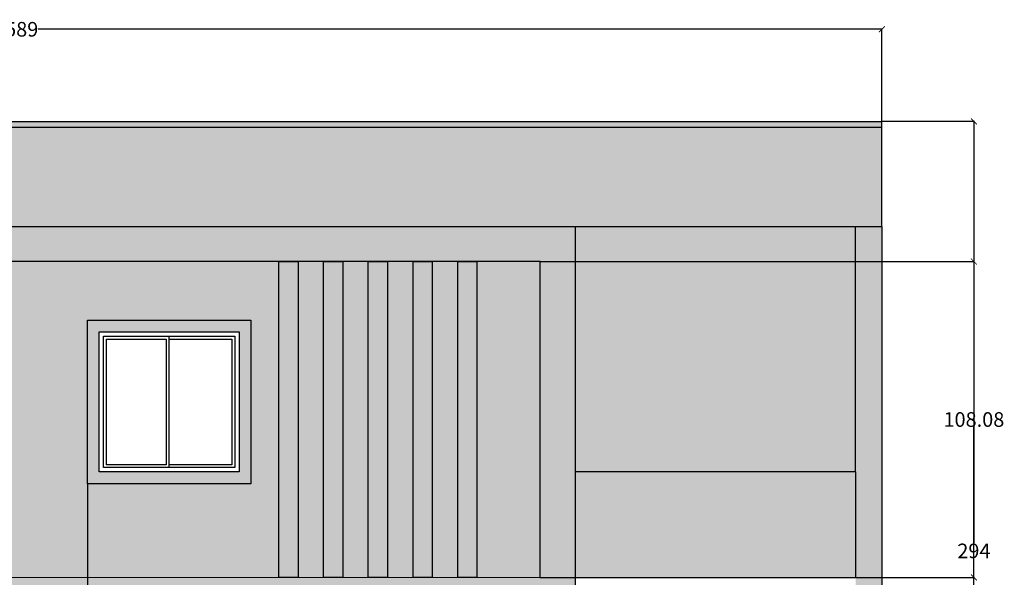
# Model space of a CAD drawing. Units: inches. Extents: x 1455 to 5994, y -182 to 2370.
# Tile 7 of 8: x 4579 to 4916, y 49 to 240. Entities that reach past the tile are written whole.
import ezdxf

# ---------------------------------------------------------------- set-up
doc = ezdxf.new("R2010")
doc.units = ezdxf.units.IN
doc.header["$MEASUREMENT"] = 0
for name, color, linetype, lineweight in [('A-ANNO-DIMS', 2, 'Continuous', 18), ('A-ELEV', 7, 'Continuous', 25), ('A-ELEV-PATT', 8, 'Continuous', 13)]:
    doc.layers.add(name, color=color, linetype=linetype, lineweight=lineweight)
doc.styles.get("Standard").update_dxf_attribs({"font": 'arial.ttf'})
doc.dimstyles.get("Standard").update_dxf_attribs({"dimtxt": 5, "dimasz": 2, "dimexe": 0.18, "dimexo": 0.0625, "dimgap": 0.09, "dimtad": 0, "dimtih": 1, "dimtoh": 1, "dimdec": 1, "dimzin": 0, "dimdsep": 46, "dimlunit": 3, "dimtxsty": 'Standard', "dimblk": 'ARCHTICK', "dimcen": 0.09, "dimadec": 0, "dimazin": 0, "dimtfac": 1, "dimtdec": 1, "dimtofl": 0, "dimtmove": 0, "dimatfit": 3, "dimfxl": 1, "dimtolj": 1, "dimtzin": 0, "dimarcsym": 0})

# ---------------------------------------------------------------- blocks, each defined once
blk = doc.blocks.new('*U8')
for p, q in [((1.5, 1.5), (1.5, 46.5)), ((1.5, 46.5), (24, 46.5)), ((24, 1.5), (24, 46.5)), ((24, 46.5), (46.5, 46.5)), ((46.5, 46.5), (46.5, 1.5)), ((24, 1.5), (1.5, 1.5)), ((46.5, 1.5), (24, 1.5))]:
    blk.add_line(p, q)
blk.add_lwpolyline([(0, 0), (0, 48), (48, 48), (48, 0)], close=True)
for points in [[(23, 45.5), (23, 2.5), (2.5, 2.5), (2.5, 45.5), (23, 45.5)], [(24, 45.5), (45.5, 45.5), (45.5, 2.5), (24, 2.5)]]:
    blk.add_lwpolyline(points)
blk = doc.blocks.new('_ArchTick')
at = {"color": 0, "linetype": 'ByBlock', "const_width": 0.15}
blk.add_lwpolyline([(-0.5, -0.5), (0.5, 0.5)], dxfattribs=at)
blk = doc.blocks.new('*D84')
at = {"layer": 'A-ANNO-DIMS', "color": 0, "lineweight": -2, "transparency": 16777216}
for p, q in [((4873.75, 205.1), (4905.37, 205.1)), ((4905.19, 205.1), (4905.19, 60.74)), ((4905.19, -88.9), (4905.19, 55.45)), ((4873.75, -88.9), (4905.37, -88.9))]:
    blk.add_line(p, q, dxfattribs=at)
at = {"layer": 'Defpoints', "color": 0, "lineweight": 25, "transparency": 16777216}
for p in [(4873.69, 205.1), (4905.19, 205.1), (4873.69, -88.9)]:
    blk.add_point(p, dxfattribs=at)
at = {"layer": 'A-ANNO-DIMS', "color": 0, "lineweight": -2, "transparency": 16777216, "xscale": 2, "yscale": 2, "zscale": 2}
for p, rotation in [((4905.19, 205.1), 90), ((4905.19, -88.9), 270)]:
    blk.add_blockref('_ArchTick', p, dxfattribs=dict(at, rotation=rotation))
at = {"layer": 'A-ANNO-DIMS', "color": 0, "transparency": 16777216, "insert": (4905.19, 58.1), "char_height": 5, "attachment_point": 5}
blk.add_mtext('\\A1;294', dxfattribs=at)
blk = doc.blocks.new('*D86')
at = {"layer": 'A-ANNO-DIMS', "color": 0, "lineweight": -2, "transparency": 16777216}
for p, q in [((4284.69, 205.16), (4284.69, 236.78)), ((4284.69, 236.6), (4573.57, 236.6)), ((4873.69, 236.6), (4584.81, 236.6)), ((4873.69, 205.16), (4873.69, 236.78))]:
    blk.add_line(p, q, dxfattribs=at)
at = {"layer": 'Defpoints', "color": 0, "lineweight": 25, "transparency": 16777216}
for p in [(4873.69, 236.6), (4284.69, 205.1), (4873.69, 205.1)]:
    blk.add_point(p, dxfattribs=at)
at = {"layer": 'A-ANNO-DIMS', "color": 0, "lineweight": -2, "transparency": 16777216, "xscale": 2, "yscale": 2, "zscale": 2, "rotation": 180}
blk.add_blockref('_ArchTick', (4284.69, 236.6), dxfattribs=at)
at = {"layer": 'A-ANNO-DIMS', "color": 0, "lineweight": -2, "transparency": 16777216, "xscale": 2, "yscale": 2, "zscale": 2}
blk.add_blockref('_ArchTick', (4873.69, 236.6), dxfattribs=at)
at = {"layer": 'A-ANNO-DIMS', "color": 0, "transparency": 16777216, "insert": (4579.19, 236.6), "char_height": 5, "attachment_point": 5}
blk.add_mtext('\\A1;589', dxfattribs=at)
blk = doc.blocks.new('*D89')
at = {"layer": 'A-ANNO-DIMS', "color": 0, "lineweight": -2, "transparency": 16777216}
for p, q in [((4396.19, 81.03), (4396.19, -120.58)), ((4601.69, 81.03), (4601.69, -120.58)), ((4396.19, -120.4), (4490.35, -120.4)), ((4601.69, -120.4), (4507.53, -120.4))]:
    blk.add_line(p, q, dxfattribs=at)
at = {"layer": 'Defpoints', "color": 0, "lineweight": 25, "transparency": 16777216}
for p in [(4396.19, 81.1), (4601.69, 81.1), (4601.69, -120.4)]:
    blk.add_point(p, dxfattribs=at)
at = {"layer": 'A-ANNO-DIMS', "color": 0, "lineweight": -2, "transparency": 16777216, "xscale": 2, "yscale": 2, "zscale": 2, "rotation": 180}
blk.add_blockref('_ArchTick', (4396.19, -120.4), dxfattribs=at)
at = {"layer": 'A-ANNO-DIMS', "color": 0, "lineweight": -2, "transparency": 16777216, "xscale": 2, "yscale": 2, "zscale": 2}
blk.add_blockref('_ArchTick', (4601.69, -120.4), dxfattribs=at)
at = {"layer": 'A-ANNO-DIMS', "color": 0, "transparency": 16777216, "insert": (4498.94, -120.4), "char_height": 5, "attachment_point": 5}
blk.add_mtext('\\A1;205.5', dxfattribs=at)
blk = doc.blocks.new('*D90')
at = {"layer": 'A-ANNO-DIMS', "color": 0, "lineweight": -2, "transparency": 16777216}
for p, q in [((4601.69, 81.03), (4601.69, -120.58)), ((4619.69, -4.97), (4619.69, -120.58)), ((4601.69, -120.4), (4607.25, -120.4)), ((4619.69, -120.4), (4614.13, -120.4))]:
    blk.add_line(p, q, dxfattribs=at)
at = {"layer": 'Defpoints', "color": 0, "lineweight": 25, "transparency": 16777216}
for p in [(4601.69, 81.1), (4619.69, -4.9), (4619.69, -120.4)]:
    blk.add_point(p, dxfattribs=at)
at = {"layer": 'A-ANNO-DIMS', "color": 0, "lineweight": -2, "transparency": 16777216, "xscale": 2, "yscale": 2, "zscale": 2, "rotation": 180}
blk.add_blockref('_ArchTick', (4601.69, -120.4), dxfattribs=at)
at = {"layer": 'A-ANNO-DIMS', "color": 0, "lineweight": -2, "transparency": 16777216, "xscale": 2, "yscale": 2, "zscale": 2}
blk.add_blockref('_ArchTick', (4619.69, -120.4), dxfattribs=at)
at = {"layer": 'A-ANNO-DIMS', "color": 0, "transparency": 16777216, "insert": (4610.69, -120.4), "char_height": 5, "attachment_point": 5}
blk.add_mtext('\\A1;18', dxfattribs=at)
blk = doc.blocks.new('*D116')
at = {"layer": 'A-ANNO-DIMS', "color": 0, "lineweight": -2, "transparency": 16777216}
for p, q in [((4756.75, 157.1), (4905.37, 157.1)), ((4905.19, 157.1), (4905.19, 105.7)), ((4905.19, 49.01), (4905.19, 100.41)), ((4756.75, 49.01), (4905.37, 49.01))]:
    blk.add_line(p, q, dxfattribs=at)
at = {"layer": 'Defpoints', "color": 0, "lineweight": 25, "transparency": 16777216}
for p in [(4756.69, 157.1), (4905.19, 157.1), (4756.69, 49.01)]:
    blk.add_point(p, dxfattribs=at)
at = {"layer": 'A-ANNO-DIMS', "color": 0, "lineweight": -2, "transparency": 16777216, "xscale": 2, "yscale": 2, "zscale": 2}
for p, rotation in [((4905.19, 157.1), 90), ((4905.19, 49.01), 270)]:
    blk.add_blockref('_ArchTick', p, dxfattribs=dict(at, rotation=rotation))
at = {"layer": 'A-ANNO-DIMS', "color": 0, "transparency": 16777216, "insert": (4905.19, 103.06), "char_height": 5, "attachment_point": 5}
blk.add_mtext('\\A1;108.08', dxfattribs=at)

msp = doc.modelspace()

# ---------------------------------------------------------------- hatches: boundary and pattern name
at = {"layer": 'A-ELEV-PATT', "transparency": 33554641}
h = msp.add_hatch(color=256, dxfattribs=at)
h.dxf.hatch_style = 1
h.paths.add_polyline_path([(4873.6884, 205.0969), (4284.6884, 205.0969), (4284.6884, 203.0969), (4873.6884, 203.0969)])
h = msp.add_hatch(color=256, dxfattribs=at)
h.dxf.hatch_style = 1
h.paths.add_polyline_path([(4873.6884, 203.0969), (4284.6884, 203.0969), (4284.6884, 169.0969), (4768.6884, 169.0969), (4864.6884, 169.0969), (4873.6884, 169.0969)])
h = msp.add_hatch(color=256, dxfattribs=at)
h.dxf.hatch_style = 1
h.paths.add_polyline_path([(4768.6884, 169.0969), (4284.6884, 169.0969), (4276.6884, 169.0969), (4276.6884, 157.0969), (4756.6884, 157.0969), (4756.6884, 49.0187), (4719.7422, 49.0288), (4719.7422, 49.0261), (4713.167, 49.0261), (4704.4367, 49.0287), (4704.4367, 49.0261), (4697.8615, 49.0261), (4689.1312, 49.0288), (4689.1312, 49.0261), (4682.556, 49.0261), (4673.8258, 49.029), (4673.8258, 49.0261), (4667.2505, 49.0261), (4471.4513, 49.0969), (4284.6884, 49.0969), (4276.6884, 49.0969), (4276.6884, 37.0915), (4543.7991, 37.0915), (4768.6843, 37.0146)])
h = msp.add_hatch(color=256, dxfattribs=at)
h.dxf.hatch_style = 1
h.paths.add_polyline_path([(4873.6884, 169.0969), (4864.6884, 169.0969), (4864.6884, 85.0969), (4864.6884, 49.0146), (4864.6884, 43.0969), (4864.6884, -70.9031), (4864.6884, -76.9031), (4861.6884, -76.9031), (4837.6884, -76.9031), (4834.6884, -76.9031), (4768.6884, -76.9031), (4763.6884, -76.9031), (4284.6884, -76.9031), (4284.6884, -88.9031), (4873.6884, -88.9031)])
h = msp.add_hatch(color=256, dxfattribs=at)
h.dxf.hatch_style = 1
h.paths.add_polyline_path([(4756.6884, 157.0969), (4735.0477, 157.0969), (4735.0477, 49.0246), (4756.6884, 49.0187)])
h.paths.add_polyline_path([(4728.4725, 157.0969), (4719.7422, 157.0969), (4719.7422, 49.0288), (4728.4725, 49.0264)])
h.paths.add_polyline_path([(4713.167, 157.0969), (4704.4367, 157.0969), (4704.4367, 49.033), (4713.167, 49.0306)])
h.paths.add_polyline_path([(4697.8615, 157.0969), (4689.1312, 157.0969), (4689.1312, 49.0372), (4697.8615, 49.0348)])
h.paths.add_polyline_path([(4682.556, 157.0969), (4673.8258, 157.0969), (4673.8258, 49.0414), (4682.556, 49.039)])
h.paths.add_polyline_path([(4864.6884, 169.0969), (4768.6884, 169.0969), (4768.6858, 85.0969), (4864.6884, 85.0969)])
h = msp.add_hatch(color=256, dxfattribs=at)
h.dxf.hatch_style = 1
h.paths.add_polyline_path([(4471.4513, 157.0969), (4284.6884, 157.0969), (4284.6884, 49.0969), (4471.4513, 49.0969), (4471.4513, 85.0969)])
h.paths.add_polyline_path([(4396.1884, 85.0969), (4396.1884, 81.0969), (4344.1884, 81.0969), (4340.1884, 81.0969), (4340.1884, 137.0969), (4344.1884, 137.0969), (4392.1884, 137.0969), (4396.1884, 137.0969)], flags=16)
h.paths.add_polyline_path([(4607.6884, 37.0697), (4543.7991, 37.0915), (4284.6884, 37.0915), (4284.6884, -76.9031), (4607.6884, -76.9031)])
h.paths.add_polyline_path([(4381.6884, -40.9031), (4381.6884, -44.9031), (4329.6884, -44.9031), (4325.6884, -44.9031), (4325.6884, 11.0969), (4329.6884, 11.0969), (4377.6884, 11.0969), (4381.6884, 11.0969)], flags=16)
h.paths.add_polyline_path([(4377.6884, -40.9031), (4329.6884, -40.9031), (4329.6884, 7.0969), (4377.6884, 7.0969)], flags=0)
h.paths.add_polyline_path([(4376.1884, -39.4031), (4353.6884, -39.4031), (4331.1884, -39.4031), (4331.1884, 5.5969), (4353.6884, 5.5969), (4376.1884, 5.5969)], flags=0)
h.paths.add_polyline_path([(4375.1884, -38.4031), (4353.6884, -38.4031), (4353.6884, 4.5969), (4375.1884, 4.5969)], flags=0)
h.paths.add_polyline_path([(4352.6884, -38.4031), (4332.1884, -38.4031), (4332.1884, 4.5969), (4352.6884, 4.5969)], flags=0)
h.paths.add_polyline_path([(4667.2505, 157.0969), (4543.8032, 157.0969), (4543.8032, 85.0969), (4543.8032, 49.0771), (4667.2505, 49.0432)])
h.paths.add_polyline_path([(4601.6884, 81.0969), (4601.6884, 137.0969), (4605.6884, 137.0969), (4653.6884, 137.0969), (4657.6884, 137.0969), (4657.6884, 81.0969)], flags=16)
h.paths.add_polyline_path([(4543.8032, 157.0969), (4471.4513, 157.0969), (4471.4513, 85.0969), (4543.8032, 85.0969)])
h.paths.add_polyline_path([(4763.6884, 37.0163), (4619.6884, 37.0656), (4619.6884, -4.9031), (4643.6884, -4.9031), (4667.6884, -4.9031), (4667.6884, -76.9031), (4763.6884, -76.9031)])
h.paths.add_polyline_path([(4864.6884, 43.0969), (4768.6884, 43.0969), (4768.6884, -76.9031), (4834.6884, -76.9031), (4834.6884, -4.9031), (4864.6884, -4.9031)])
h = msp.add_hatch(color=256, dxfattribs=at)
h.dxf.hatch_style = 1
h.paths.add_polyline_path([(4735.0477, 157.0969), (4728.4725, 157.0969), (4728.4725, 49.0283), (4735.0477, 49.0261)])
h.paths.add_polyline_path([(4719.7422, 157.0969), (4713.167, 157.0969), (4713.167, 49.0336), (4719.7422, 49.0313)])
h.paths.add_polyline_path([(4704.4367, 157.0969), (4697.8615, 157.0969), (4697.8615, 49.0388), (4704.4367, 49.0366)])
h.paths.add_polyline_path([(4689.1312, 157.0969), (4682.556, 157.0969), (4682.556, 49.0441), (4689.1312, 49.0418)])
h.paths.add_polyline_path([(4673.8258, 157.0969), (4667.2505, 157.0969), (4667.2505, 49.0493), (4673.8258, 49.047)])
h = msp.add_hatch(color=256, dxfattribs=at)
h.dxf.hatch_style = 1
h.paths.add_polyline_path([(4396.1884, 137.0969), (4392.1884, 137.0969), (4344.1884, 137.0969), (4340.1884, 137.0969), (4340.1884, 81.0969), (4344.1884, 81.0969), (4396.1884, 81.0969), (4396.1884, 85.0969)])
h.paths.add_polyline_path([(4344.1884, 133.0969), (4392.1884, 133.0969), (4392.1884, 85.0969), (4344.1884, 85.0969)], flags=16)
h.paths.add_polyline_path([(4345.6884, 131.5969), (4368.1884, 131.5969), (4390.6884, 131.5969), (4390.6884, 86.5969), (4368.1884, 86.5969), (4345.6884, 86.5969)], flags=0)
h.paths.add_polyline_path([(4346.6884, 130.5969), (4367.1884, 130.5969), (4367.1884, 87.5969), (4346.6884, 87.5969)], flags=0)
h.paths.add_polyline_path([(4368.1884, 130.5969), (4389.6884, 130.5969), (4389.6884, 87.5969), (4368.1884, 87.5969)], flags=0)
h.paths.add_polyline_path([(4657.6884, 137.0969), (4653.6884, 137.0969), (4605.6884, 137.0969), (4601.6884, 137.0969), (4601.6884, 81.0969), (4657.6884, 81.0969)])
h.paths.add_polyline_path([(4653.6884, 133.0969), (4653.6884, 85.0969), (4605.6884, 85.0969), (4605.6884, 133.0969)], flags=16)
h.paths.add_polyline_path([(4629.6884, 131.5969), (4652.1884, 131.5969), (4652.1884, 86.5969), (4629.6884, 86.5969), (4607.1884, 86.5969), (4607.1884, 131.5969)], flags=0)
h.paths.add_polyline_path([(4628.6884, 130.5969), (4628.6884, 87.5969), (4608.1884, 87.5969), (4608.1884, 130.5969)], flags=0)
h.paths.add_polyline_path([(4629.6884, 130.5969), (4651.1884, 130.5969), (4651.1884, 87.5969), (4629.6884, 87.5969)], flags=0)
h.paths.add_polyline_path([(4381.6884, 11.0969), (4377.6884, 11.0969), (4329.6884, 11.0969), (4325.6884, 11.0969), (4325.6884, -44.9031), (4329.6884, -44.9031), (4381.6884, -44.9031), (4381.6884, -40.9031)])
h.paths.add_polyline_path([(4377.6884, 7.0969), (4377.6884, -40.9031), (4329.6884, -40.9031), (4329.6884, 7.0969)], flags=16)
h.paths.add_polyline_path([(4353.6884, 5.5969), (4376.1884, 5.5969), (4376.1884, -39.4031), (4353.6884, -39.4031), (4331.1884, -39.4031), (4331.1884, 5.5969)], flags=0)
h.paths.add_polyline_path([(4353.6884, 4.5969), (4375.1884, 4.5969), (4375.1884, -38.4031), (4353.6884, -38.4031)], flags=0)
h.paths.add_polyline_path([(4352.6884, -38.4031), (4332.1884, -38.4031), (4332.1884, 4.5969), (4352.6884, 4.5969)], flags=0)
at = {"layer": 'A-ELEV-PATT', "transparency": 33554666}
h = msp.add_hatch(color=256, dxfattribs=at)
h.dxf.hatch_style = 1
h.paths.add_polyline_path([(4864.6884, 85.0969), (4768.6884, 85.0969), (4768.6884, 49.0969), (4864.6884, 49.0969)])
h.paths.add_polyline_path([(4543.8032, 85.0969), (4471.4513, 85.0969), (4471.4513, 49.0969), (4543.8032, 49.0969)])

# ---------------------------------------------------------------- linework, layer by layer
at = {"layer": 'A-ELEV'}
for p, q in [((4284.6884, 205.0969), (4873.6884, 205.0969)), ((4284.6884, 203.0969), (4873.6884, 203.0969)), ((4873.6884, 169.0969), (4873.6884, 205.0969)), ((4768.6884, 169.0969), (4864.6884, 169.0969)), ((4864.6884, 85.0969), (4864.6884, 169.0969)), ((4864.6884, 169.0969), (4873.6884, 169.0969)), ((4873.6884, 169.0969), (4873.6884, -88.9031)), ((4601.6884, 81.0969), (4601.6884, 137.0969)), ((4601.6884, 137.0969), (4605.6884, 137.0969)), ((4605.6884, 137.0969), (4653.6884, 137.0969)), ((4653.6884, 137.0969), (4657.6884, 137.0969)), ((4657.6884, 137.0969), (4657.6884, 81.0969)), ((4653.6884, 85.0969), (4605.6884, 85.0969)), ((4864.6884, 85.0969), (4768.6884, 85.0969)), ((4864.6884, 85.0969), (4864.6884, 49.0146)), ((4657.6884, 81.0969), (4601.6884, 81.0969))]:
    msp.add_line(p, q, dxfattribs=at)
msp.add_lwpolyline([(4756.6884, 49.0146), (4756.6884, 157.0969), (4276.6884, 157.0969), (4276.6884, 169.0969), (4284.6884, 169.0969), (4768.6884, 169.0969), (4768.6843, 37.0146), (4543.7991, 37.0915), (4276.6884, 37.0915), (4276.6884, 49.0969), (4284.6884, 49.0969), (4471.4513, 49.0969), (4756.6884, 49.0187)], dxfattribs=at)
for points in [[(4667.2505, 157.0969), (4673.8258, 157.0969), (4673.8258, 49.0261), (4667.2505, 49.0261)], [(4682.556, 157.0969), (4689.1312, 157.0969), (4689.1312, 49.0261), (4682.556, 49.0261)], [(4697.8615, 157.0969), (4704.4367, 157.0969), (4704.4367, 49.0261), (4697.8615, 49.0261)], [(4713.167, 157.0969), (4719.7422, 157.0969), (4719.7422, 49.0261), (4713.167, 49.0261)], [(4728.4725, 157.0969), (4735.0477, 157.0969), (4735.0477, 49.0261), (4728.4725, 49.0261)]]:
    msp.add_lwpolyline(points, close=True, dxfattribs=at)

# ---------------------------------------------------------------- block references
msp.add_blockref('*U8', (4605.6884, 85.0969), dxfattribs=at)

# ---------------------------------------------------------------- dimensions: what is measured, and where the dimension line sits
at = {"layer": 'A-ANNO-DIMS'}
for base, p1, p2, override, picture, middle in [((4873.6884, 236.5969), (4284.6884, 205.0969), (4873.6884, 205.0969), {"dimdec": 0, "dimlfac": 1, "dimrnd": 0, "dimzin": 0, "dimdsep": 46, "dimlunit": 2}, '*D86', (4579.1884, 236.5969)), ((4601.6884, -120.4031), (4396.1884, 81.0969), (4601.6884, 81.0969), {"dimdec": 1, "dimlfac": 1, "dimrnd": 0, "dimzin": 0, "dimdsep": 46, "dimlunit": 2}, '*D89', (4498.9384, -120.4031)), ((4619.6884, -120.4031), (4601.6884, 81.0969), (4619.6884, -4.9031), {"dimdec": 0, "dimlfac": 1, "dimrnd": 0, "dimzin": 0, "dimdsep": 46, "dimlunit": 2}, '*D90', (4610.6884, -120.4031))]:
    dim = msp.add_linear_dim(base=base, p1=p1, p2=p2, dimstyle='Standard', override=override, dxfattribs=at)
    dim.commit()
    dim.dimension.update_dxf_attribs({"geometry": picture, "text_midpoint": middle})
for base, p1, p2, override, picture, middle in [((4905.1884, 205.0969), (4873.6884, -88.9031), (4873.6884, 205.0969), {"dimdec": 0, "dimlfac": 1, "dimrnd": 0, "dimzin": 0, "dimdsep": 46, "dimlunit": 2}, '*D84', (4905.1884, 58.0969)), ((4905.1884, 157.0969), (4756.6884, 49.0146), (4756.6884, 157.0969), {"dimdec": 2, "dimlfac": 1, "dimrnd": 0, "dimzin": 0, "dimdsep": 46, "dimlunit": 2}, '*D116', (4905.1884, 103.0558))]:
    dim = msp.add_linear_dim(base=base, p1=p1, p2=p2, angle=90, dimstyle='Standard', override=override, dxfattribs=at)
    dim.commit()
    dim.dimension.update_dxf_attribs({"geometry": picture, "text_midpoint": middle})

doc.saveas('drawing.dxf')
